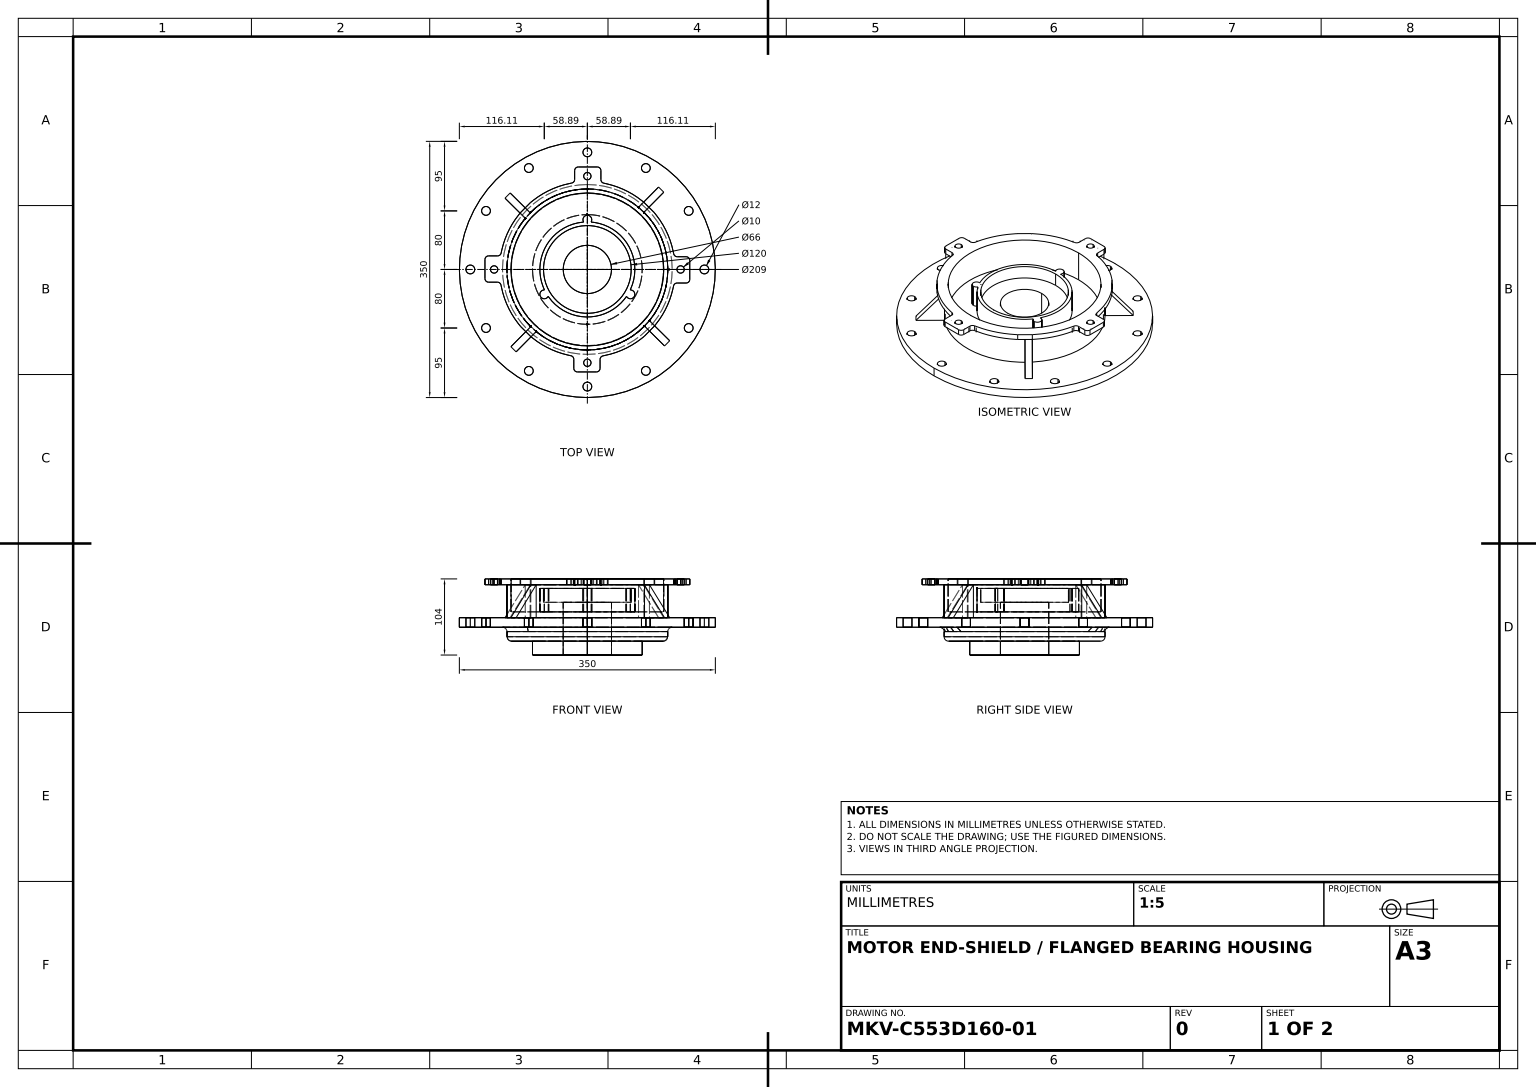
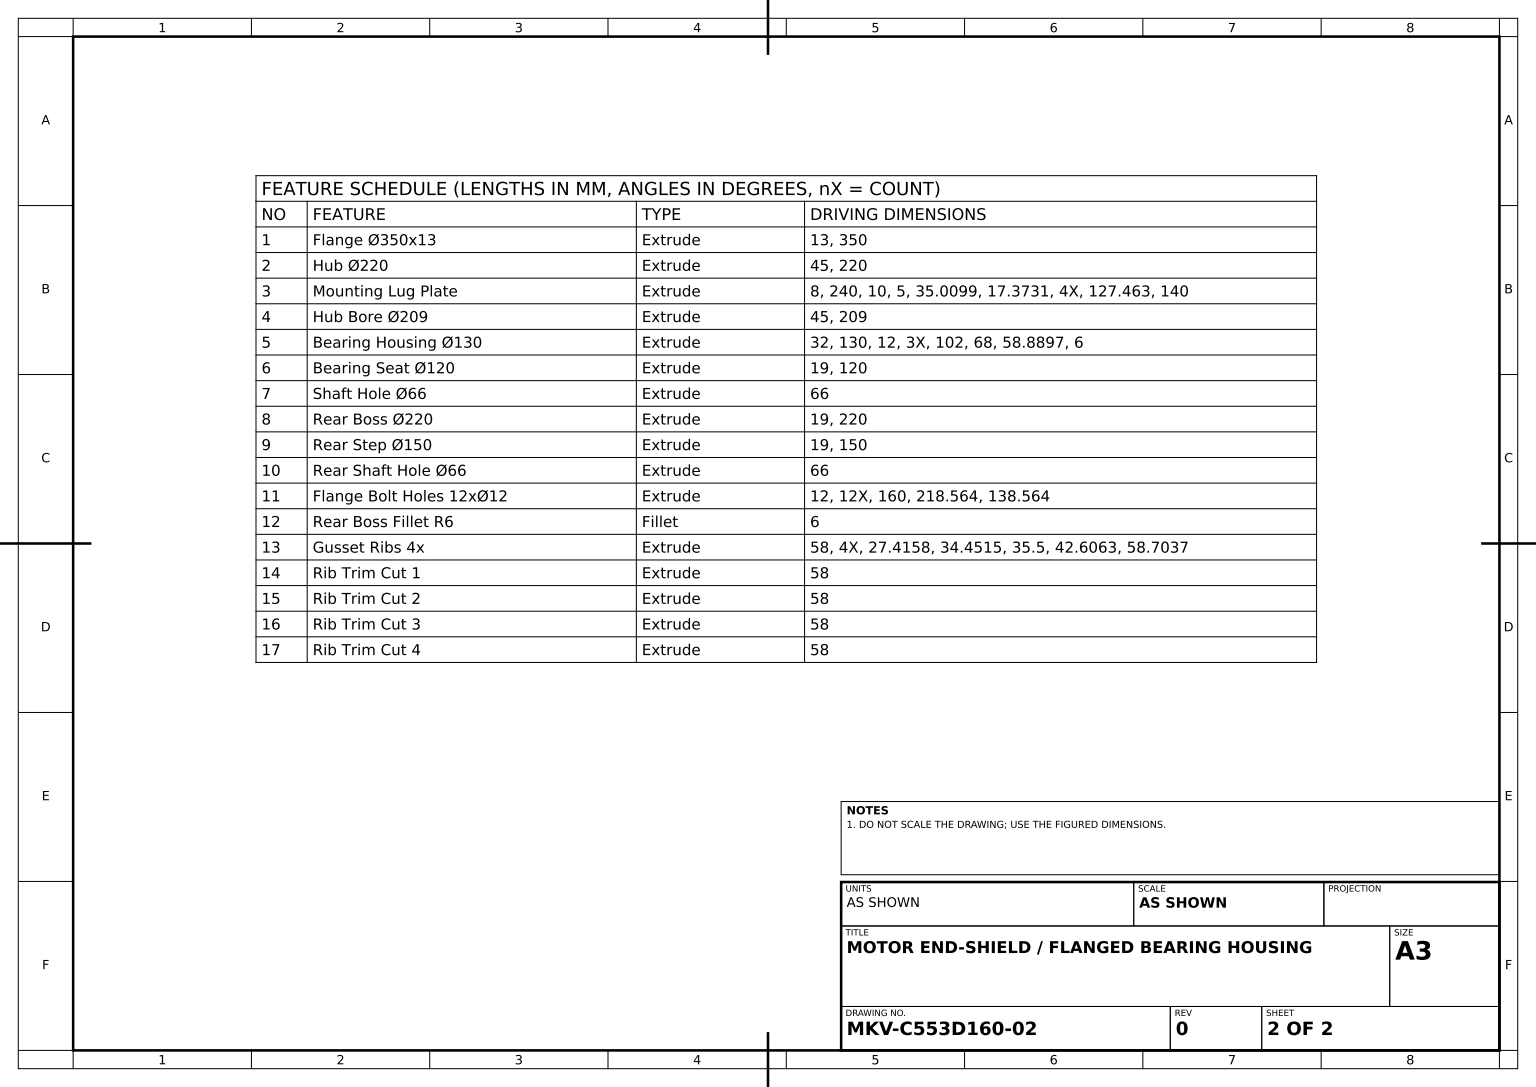
from build123d import *

# Parameters (mm, degrees)
FLANGE_SKETCH_R                = 175
FLANGE_350X13_DEPTH            = 13
HUB_SKETCH_R                   = 110
HUB_220_DEPTH                  = 45
LUG_PLATE_SKETCH_R             = 5
MOUNTING_LUG_PLATE_DEPTH       = 8
HUB_BORE_SKETCH_R              = 104.5
HUB_BORE_209_DEPTH             = 45
BEARING_HOUSING_130_DEPTH      = 32
BEARING_SEAT_SKETCH_R          = 60
BEARING_SEAT_120_DEPTH         = 19
SHAFT_HOLE_SKETCH_R            = 33
SHAFT_HOLE_66_DEPTH            = 250.811929259
REAR_START                     = 19
REAR_BOSS_SKETCH_R             = 110
REAR_BOSS_220_DEPTH            = 19
REAR_STEP_SKETCH_R             = 75
REAR_STEP_150_DEPTH            = 19
REAR_SHAFT_HOLE_SKETCH_R       = 33
REAR_SHAFT_HOLE_66_DEPTH       = 269.451112868
FLANGE_BOLT_HOLES_SKETCH_R     = 6
FLANGE_BOLT_HOLES_12X_12_DEPTH = 254.09879494
REAR_BOSS_FILLET_R6_R          = 6
GUSSET_RIBS_4X_DEPTH           = 58
RIB_TRIM_CUT_1_DEPTH           = 58
RIB_TRIM_CUT_2_DEPTH           = 58
RIB_TRIM_CUT_3_DEPTH           = 58
RIB_TRIM_CUT_4_DEPTH           = 58


with BuildPart() as part:
    # Flange Sketch → Flange Ø350x13 (new body)
    with BuildSketch(Plane(origin=(0, 0, 0), x_dir=(1, 0, 0), z_dir=(0, 1, 0))):
        with Locations(Location((0, 0, 0), (0, 0, 90))):
            Circle(FLANGE_SKETCH_R)
    extrude(amount=FLANGE_350X13_DEPTH)

    # Hub Sketch → Hub Ø220 (add)
    with BuildSketch(Plane(origin=(0, 13, 0), x_dir=(1, 0, 0), z_dir=(0, 1, 0))):
        with Locations(Location((0, 0, 0), (0, 0, 90))):
            Circle(HUB_SKETCH_R)
    extrude(amount=HUB_220_DEPTH)

    # Lug Plate Sketch → Mounting Lug Plate (add)
    with BuildSketch(Plane(origin=(0, 58, 0), x_dir=(1, 0, 0), z_dir=(0, 1, 0))):
        with BuildLine():
            Line((122.981475637, 17.37312339), (135, 17.37312339))
            ThreePointArc((135, 17.37312339), (138.535533906, 15.908657296), (140, 12.37312339))
            Line((140, 12.37312339), (140, -13.53168384))
            ThreePointArc((140, -13.53168384), (138.535533906, -17.067217746), (135, -18.53168384))
            Line((135, -18.53168384), (122.765059588, -18.53168384))
            ThreePointArc((122.765059588, -18.53168384), (119.579650412, -19.677702991), (117.854457205, -22.590416486))
            ThreePointArc((117.854457205, -22.590416486), (84.451840643, -85.251900929), (21.478198454, -118.062216611))
            ThreePointArc((21.478198454, -118.062216611), (18.534202664, -119.777932651), (17.37312339, -122.981475637))
            Line((17.37312339, -122.981475637), (17.37312339, -135))
            ThreePointArc((17.37312339, -135), (15.908657296, -138.535533906), (12.37312339, -140))
            Line((12.37312339, -140), (-13.53168384, -140))
            ThreePointArc((-13.53168384, -140), (-17.067217746, -138.535533906), (-18.53168384, -135))
            Line((-18.53168384, -135), (-18.53168384, -122.765059588))
            ThreePointArc((-18.53168384, -122.765059588), (-19.677702991, -119.579650412), (-22.590416486, -117.854457205))
            ThreePointArc((-22.590416486, -117.854457205), (-85.251900929, -84.451840643), (-118.062216611, -21.478198454))
            ThreePointArc((-118.062216611, -21.478198454), (-119.777932651, -18.534202664), (-122.981475637, -17.37312339))
            Line((-122.981475637, -17.37312339), (-135, -17.37312339))
            ThreePointArc((-135, -17.37312339), (-138.535533906, -15.908657296), (-140, -12.37312339))
            Line((-140, -12.37312339), (-140, 13.53168384))
            ThreePointArc((-140, 13.53168384), (-138.535533906, 17.067217746), (-135, 18.53168384))
            Line((-135, 18.53168384), (-122.765059588, 18.53168384))
            ThreePointArc((-122.765059588, 18.53168384), (-119.579650412, 19.677702991), (-117.854457205, 22.590416486))
            ThreePointArc((-117.854457205, 22.590416486), (-84.451840643, 85.251900929), (-21.478198454, 118.062216611))
            ThreePointArc((-21.478198454, 118.062216611), (-18.534202664, 119.777932651), (-17.37312339, 122.981475637))
            Line((-17.37312339, 122.981475637), (-17.37312339, 135))
            ThreePointArc((-17.37312339, 135), (-15.908657296, 138.535533906), (-12.37312339, 140))
            Line((-12.37312339, 140), (13.53168384, 140))
            ThreePointArc((13.53168384, 140), (17.067217746, 138.535533906), (18.53168384, 135))
            Line((18.53168384, 135), (18.53168384, 122.765059588))
            ThreePointArc((18.53168384, 122.765059588), (19.677702991, 119.579650412), (22.590416486, 117.854457205))
            ThreePointArc((22.590416486, 117.854457205), (85.251900929, 84.451840643), (118.062216611, 21.478198454))
            ThreePointArc((118.062216611, 21.478198454), (119.777932651, 18.534202664), (122.981475637, 17.37312339))
        make_face()
        with Locations(Location((0, 127.463390021, 0), (0, 0, 270))):
            Circle(LUG_PLATE_SKETCH_R, mode=Mode.SUBTRACT)
        with Locations(Location((127.463390021, 0, 0), (0, 0, 270))):
            Circle(LUG_PLATE_SKETCH_R, mode=Mode.SUBTRACT)
        with Locations(Location((0, -127.463390021, 0), (0, 0, 270))):
            Circle(LUG_PLATE_SKETCH_R, mode=Mode.SUBTRACT)
        with Locations(Location((-127.463390021, 0, 0), (0, 0, 270))):
            Circle(LUG_PLATE_SKETCH_R, mode=Mode.SUBTRACT)
    extrude(amount=MOUNTING_LUG_PLATE_DEPTH)

    # Hub Bore Sketch → Hub Bore Ø209 (cut)
    with BuildSketch(Plane(origin=(0, 66, 0), x_dir=(1, 0, 0), z_dir=(0, 1, 0))):
        with Locations(Location((0, 0, 0), (0, 0, 270))):
            Circle(HUB_BORE_SKETCH_R)
    extrude(amount=-HUB_BORE_209_DEPTH, mode=Mode.SUBTRACT)

    # Bearing Housing Sketch → Bearing Housing Ø130 (add)
    with BuildSketch(Plane(origin=(0, 21, 0), x_dir=(1, 0, 0), z_dir=(0, 1, 0))):
        with BuildLine():
            ThreePointArc((-5.076357907, 64.801470588), (-56.291651246, 32.5), (-58.657898686, -28.004480388))
            ThreePointArc((-58.657898686, -28.004480388), (-64.08587988, -37), (-53.581540778, -36.7969902))
            ThreePointArc((-53.581540778, -36.7969902), (0, -65), (53.581540778, -36.7969902))
            ThreePointArc((53.581540778, -36.7969902), (64.08587988, -37), (58.657898686, -28.004480388))
            ThreePointArc((58.657898686, -28.004480388), (56.291651246, 32.5), (5.076357907, 64.801470588))
            ThreePointArc((5.076357907, 64.801470588), (0, 74), (-5.076357907, 64.801470588))
        make_face()
    extrude(amount=BEARING_HOUSING_130_DEPTH)

    # Bearing Seat Sketch → Bearing Seat Ø120 (cut)
    with BuildSketch(Plane(origin=(0, 53, 0), x_dir=(1, 0, 0), z_dir=(0, 1, 0))):
        with Locations(Location((0, 0, 0), (0, 0, 270))):
            Circle(BEARING_SEAT_SKETCH_R)
    extrude(amount=-BEARING_SEAT_120_DEPTH, mode=Mode.SUBTRACT)

    # Shaft Hole Sketch → Shaft Hole Ø66 (cut, through all)
    with BuildSketch(Plane(origin=(0, 34, 0), x_dir=(1, 0, 0), z_dir=(0, 1, 0))):
        with Locations(Location((0, 0, 0), (0, 0, 270))):
            Circle(SHAFT_HOLE_SKETCH_R)
    extrude(amount=-SHAFT_HOLE_66_DEPTH, mode=Mode.SUBTRACT)

    # Rear Boss Sketch → Rear Boss Ø220 (add)
    with BuildSketch(Plane.XZ.offset(REAR_START)):
        with Locations(Location((0, 0, 0), (0, 0, 270))):
            Circle(REAR_BOSS_SKETCH_R)
    extrude(amount=-REAR_BOSS_220_DEPTH)

    # Rear Step Sketch → Rear Step Ø150 (add)
    with BuildSketch(Plane.XZ.offset(19)):
        with Locations(Location((0, 0, 0), (0, 0, 270))):
            Circle(REAR_STEP_SKETCH_R)
    extrude(amount=REAR_STEP_150_DEPTH)

    # Rear Shaft Hole Sketch → Rear Shaft Hole Ø66 (cut, through all)
    with BuildSketch(Plane.XZ.offset(38)):
        with Locations(Location((0, 0, 0), (0, 0, 90))):
            Circle(REAR_SHAFT_HOLE_SKETCH_R)
    extrude(amount=-REAR_SHAFT_HOLE_66_DEPTH, mode=Mode.SUBTRACT)

    # Flange Bolt Holes Sketch → Flange Bolt Holes 12xØ12 (cut, through all)
    with BuildSketch(Plane(origin=(0, 13, 0), x_dir=(1, 0, 0), z_dir=(0, 1, 0))):
        with Locations(Location((0, 160, 0), (0, 0, 270))):
            Circle(FLANGE_BOLT_HOLES_SKETCH_R)
        with Locations(Location((80, 138.564064606, 0), (0, 0, 270))):
            Circle(FLANGE_BOLT_HOLES_SKETCH_R)
        with Locations(Location((138.564064606, 80, 0), (0, 0, 270))):
            Circle(FLANGE_BOLT_HOLES_SKETCH_R)
        with Locations(Location((160, 0, 0), (0, 0, 270))):
            Circle(FLANGE_BOLT_HOLES_SKETCH_R)
        with Locations(Location((138.564064606, -80, 0), (0, 0, 270))):
            Circle(FLANGE_BOLT_HOLES_SKETCH_R)
        with Locations(Location((80, -138.564064606, 0), (0, 0, 270))):
            Circle(FLANGE_BOLT_HOLES_SKETCH_R)
        with Locations(Location((0, -160, 0), (0, 0, 270))):
            Circle(FLANGE_BOLT_HOLES_SKETCH_R)
        with Locations(Location((-80, -138.564064606, 0), (0, 0, 270))):
            Circle(FLANGE_BOLT_HOLES_SKETCH_R)
        with Locations(Location((-138.564064605, -80, 0), (0, 0, 270))):
            Circle(FLANGE_BOLT_HOLES_SKETCH_R)
        with Locations(Location((-160, 0, 0), (0, 0, 270))):
            Circle(FLANGE_BOLT_HOLES_SKETCH_R)
        with Locations(Location((-138.564064606, 80, 0), (0, 0, 270))):
            Circle(FLANGE_BOLT_HOLES_SKETCH_R)
        with Locations(Location((-80, 138.564064606, 0), (0, 0, 270))):
            Circle(FLANGE_BOLT_HOLES_SKETCH_R)
    extrude(amount=-FLANGE_BOLT_HOLES_12X_12_DEPTH, mode=Mode.SUBTRACT)

    # Rear Boss Fillet R6
    rear_boss_fillet_r6_edges = [part.edges().sort_by_distance(p)[0] for p in [
        (0, 0, 110),
        (0, -19, 110),
    ]]
    fillet(rear_boss_fillet_r6_edges, radius=REAR_BOSS_FILLET_R6_R)

    # Gusset Ribs Sketch → Gusset Ribs 4x (add)
    with BuildSketch(Plane(origin=(0, 66, 0), x_dir=(1, 0, 0), z_dir=(0, 1, 0))):
        Polygon((-74.260582015, 73.522894114), (-105.548494983, 104.5), (-112.584178631, 97.393724209), (-81.296265662, 66.416618323), align=None)
        Polygon((104.5, 105.548494983), (97.393724209, 112.584178631), (66.416618323, 81.296265662), (73.522894114, 74.260582015), align=None)
        Polygon((105.548494983, -104.5), (112.584178631, -97.393724209), (81.296265662, -66.416618323), (74.260582015, -73.522894114), align=None)
        Polygon((-104.5, -105.548494983), (-97.393724209, -112.584178631), (-66.416618323, -81.296265662), (-73.522894114, -74.260582015), align=None)
    extrude(amount=-GUSSET_RIBS_4X_DEPTH)

    # Rib Trim Sketch 1 → Rib Trim Cut 1 (cut)
    with BuildSketch(Plane(origin=(7.106275791, 0, 7.035683647), x_dir=(0.7035683647248037, 0, -0.7106275790865887), z_dir=(0.7106275790865887, 0, 0.7035683647248037))):
        Polygon((-109.544511501, 58), (-148.52856558, 13), (-148.52856558, 66), (-119.582607431, 66), (-119.582607431, 58), align=None)
    extrude(amount=-RIB_TRIM_CUT_1_DEPTH, mode=Mode.SUBTRACT)

    # Rib Trim Sketch 2 → Rib Trim Cut 2 (cut)
    with BuildSketch(Plane(origin=(-7.035683647, 0, 7.106275791), x_dir=(0.7106275790865887, 0, 0.7035683647248037), z_dir=(-0.7035683647248037, 0, 0.7106275790865887))):
        Polygon((-109.544511501, 58), (-148.52856558, 13), (-148.52856558, 66), (-119.582607431, 66), (-119.582607431, 58), align=None)
    extrude(amount=-RIB_TRIM_CUT_2_DEPTH, mode=Mode.SUBTRACT)

    # Rib Trim Sketch 3 → Rib Trim Cut 3 (cut)
    with BuildSketch(Plane(origin=(-7.106275791, 0, -7.035683647), x_dir=(-0.7035683647248037, 0, 0.7106275790865887), z_dir=(-0.7106275790865887, 0, -0.7035683647248037))):
        Polygon((-109.544511501, 58), (-148.52856558, 13), (-148.52856558, 66), (-119.582607431, 66), (-119.582607431, 58), align=None)
    extrude(amount=-RIB_TRIM_CUT_3_DEPTH, mode=Mode.SUBTRACT)

    # Rib Trim Sketch 4 → Rib Trim Cut 4 (cut)
    with BuildSketch(Plane(origin=(7.035683647, 0, -7.106275791), x_dir=(-0.7106275790865887, 0, -0.7035683647248037), z_dir=(0.7035683647248037, 0, -0.7106275790865887))):
        Polygon((-109.544511501, 58), (-148.52856558, 13), (-148.52856558, 66), (-119.582607431, 66), (-119.582607431, 58), align=None)
    extrude(amount=-RIB_TRIM_CUT_4_DEPTH, mode=Mode.SUBTRACT)


solid = part.part
